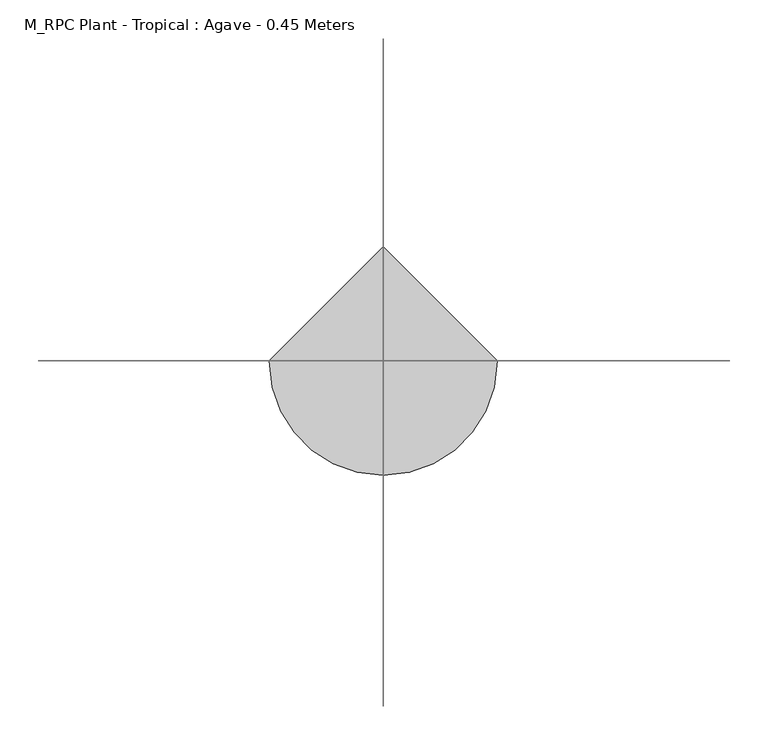
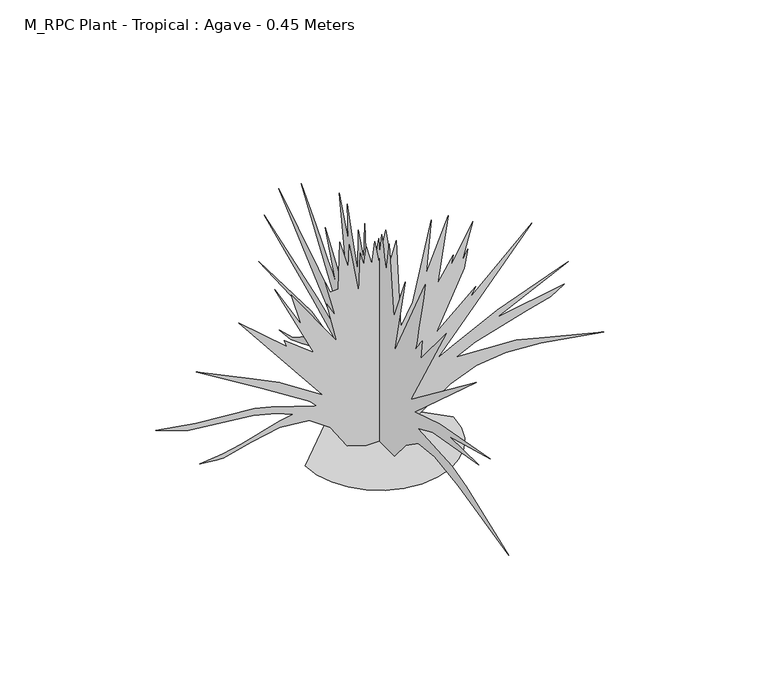
"""IFC4 building model written with IfcOpenShell, lengths in millimetres: geographic element geometry, M_RPC Plant - Tropical : Agave - 0.45 Meters."""

from ifc_helpers import new_model, si_unit, origin, place, context, project, spatial, triangles, source, transform, mapped, element, save


def m_rpc_plant_tropical_agave_0_45_meters_eb57889b(model_context):
    return source(origin(), model_context, "Body", "Tessellation", [
        triangles([(-148.1386958, 0.0, 9.3e-06), (-144.2171964, -33.9885277, 9.3e-06), (-133.048683, -65.2018023, 9.3e-06), (-115.5276685, -92.7450748, 9.3e-06), (-92.5484025, -115.7243407, 9.3e-06), (-65.0051301, -133.2453552, 9.3e-06), (-33.7918577, -144.4138686, 9.3e-06), (0.1966776, -148.335368, 9.3e-06), (34.1851976, -144.4138686, 9.3e-06), (65.3984745, -133.2453552, 9.3e-06), (92.941747, -115.7243407, 9.3e-06), (115.921013, -92.7450748, 9.3e-06), (133.4420274, -65.2018023, 9.3e-06), (144.6105409, -33.9885277, 9.3e-06), (148.5320402, 1.3e-05, 9.3e-06), (0.1966516, 148.335368, 9.3e-06), (-24.3504237, 1.1e-06, 2.5e-06), (-64.1988793, 2e-06, 12.9348607), (-97.895905, 5e-07, 64.0713026), (-140.594189, 5e-07, 94.1593235), (-198.9417449, 2.8e-06, 99.5475756), (-255.4485429, 5.9e-06, 87.7748204), (-311.5910826, 9.2e-06, 73.8080584), (-324.2335885, 9.8e-06, 74.3145591), (-359.378609, 1.11e-05, 77.950311), (-313.1035629, 8.8e-06, 82.7858171), (-277.6960585, 6.8e-06, 90.344322), (-199.7057426, 2e-06, 113.0485866), (-172.7469775, 5e-07, 117.942592), (-204.8844963, 1.2e-06, 130.9928583), (-252.5285358, 2.5e-06, 143.4918682), (-382.9561306, 7.4e-06, 157.5558808), (-447.8461741, 8.9e-06, 179.7488939), (-367.8611217, 6.2e-06, 166.4181305), (-249.0960418, 1.6e-06, 156.7231191), (-216.6905162, 6e-07, 148.7013704), (-125.4831746, -1.6e-06, 119.154591), (-138.0646922, -1.9e-06, 133.1736027), (-234.3990283, -1.3e-06, 193.9569111), (-366.6486231, -4e-07, 275.4877267), (-252.1085396, -2.1e-06, 220.5199336), (-200.6204942, -2.9e-06, 195.5036553), (-113.3644194, -3.3e-06, 138.5448591), (-281.816065, -8.5e-06, 349.4127929), (-184.8657327, -7.8e-06, 265.7927153), (-189.7134928, -8.4e-06, 280.3352324), (-131.5426794, -8.2e-06, 234.2839372), (-209.1037518, -1.44e-05, 395.4653234), (-155.7804623, -1.12e-05, 302.1502344), (-176.3827294, -1.45e-05, 372.4403117), (-85.4908937, -1.07e-05, 242.7671948), (-104.8811618, -1.49e-05, 327.6002798), (-87.9146465, -1.39e-05, 297.3027469), (-108.5169137, -1.76e-05, 374.8628019), (-97.9506527, -1.66e-05, 351.3077717), (-81.76514, -1.74e-05, 351.3277923), (-79.4313889, -2.33e-05, 450.0003668), (-62.2313759, -2.06e-05, 390.7203006), (-60.0411253, -2.35e-05, 437.880358), (-40.6511115, -1.79e-05, 330.02277), (-38.2271089, -2.29e-05, 412.4328197), (-30.9558549, -2.16e-05, 384.5578134), (-26.1083514, -2.4e-05, 422.1278312), (-15.2013409, -2.2e-05, 380.9227881), (-9.1419111, -2.5e-05, 426.9753551), (-0.6586671, -2.27e-05, 380.9227881), (12.6721065, -2.7e-05, 443.9403442), (23.5791135, -2.35e-05, 377.2877993), (34.4861967, -2.62e-05, 413.6428476), (42.9694566, -1.54e-05, 227.0126877), (67.2069761, -1.91e-05, 271.8527196), (104.0335027, -3.03e-05, 433.0253491), (93.8687435, -2.34e-05, 323.9627475), (138.4672839, -3.17e-05, 430.0728404), (116.8945182, -2.27e-05, 294.8777314), (148.4037868, -2.69e-05, 343.3552774), (143.5562902, -2.54e-05, 321.5402573), (187.1843049, -3.2e-05, 400.312811), (165.3703021, -2.65e-05, 322.7527559), (177.4890573, -2.84e-05, 345.7777677), (170.9330439, -2.58e-05, 308.0802504), (114.4707654, -1.64e-05, 190.6558953), (193.2438187, -2.4e-05, 260.9452096), (181.1248092, -2.22e-05, 240.3434511), (305.9494211, -3.46e-05, 355.4727791), (116.8945182, -1.32e-05, 136.120861), (156.175787, -1.61e-05, 155.588123), (236.8716063, -2.2e-05, 195.5036553), (378.6619886, -3.14e-05, 248.8266905), (235.6598525, -2.1e-05, 179.7488939), (371.0494809, -2.83e-05, 203.1156544), (343.871961, -2.62e-05, 186.8916447), (295.8769073, -2.33e-05, 173.2968894), (192.5770716, -1.7e-05, 143.7823665), (154.4632825, -1.42e-05, 125.2138505), (274.4393895, -1.91e-05, 119.154591), (331.2944584, -2.07e-05, 104.4295814), (450.1645283, -2.41e-05, 74.3145591), (324.0894476, -1.98e-05, 94.6895782), (253.5743659, -1.7e-05, 99.5105775), (194.5445751, -1.4e-05, 92.6238249), (142.6707883, -1.05e-05, 72.2130568), (85.3409936, -5.7e-06, 33.5950265), (32.7349455, -1.4e-06, 0.0), (0.196672, 19.7673413, 8.9e-06), (0.1966732, 47.0472873, 9.8e-06), (0.1966747, 67.3315551, 19.7666418), (0.1966772, 98.1250789, 58.1885449), (0.1966793, 130.6278551, 79.4465678), (0.1966812, 171.5303912, 83.5105639), (0.1966824, 205.2991693, 71.7218077), (0.1966844, 267.9552104, 45.114788), (0.1966857, 307.0702466, 29.8075238), (0.1966874, 347.7627846, 24.6271691), (0.1966857, 300.5702436, 38.2485284), (0.1966843, 245.8184439, 73.6468083), (0.1966827, 196.7091595, 96.1225757), (0.196681, 158.7086266, 94.9168263), (0.1966826, 185.5584048, 108.6283349), (0.1966859, 252.0827055, 120.1018443), (0.1966936, 419.0128324, 127.5108488), (0.1966855, 235.0574365, 132.4853544), (0.1966818, 162.3476305, 116.8738436), (0.1966792, 117.5043466, 94.9168263), (0.1966819, 157.4268734, 125.6566015), (0.1966862, 230.1374425, 162.6691225), (0.196696, 399.8753377, 236.7079353), (0.1966859, 214.4554237, 174.9013882), (0.1966819, 145.377618, 145.8161177), (0.1966963, 348.9752832, 323.9627475), (0.1966833, 143.900864, 195.427915), (0.1966945, 270.2027113, 382.1353231), (0.1966926, 244.8639419, 353.83527), (0.1966907, 220.4639232, 326.4102725), (0.1966889, 197.940407, 300.737748), (0.1966873, 178.2316355, 277.6927156), (0.196686, 162.2761232, 258.1477059), (0.1966851, 151.0121214, 242.9834425), (0.1966845, 145.377618, 233.0721834), (0.1966896, 187.793897, 339.7177814), (0.196686, 146.5683701, 279.2777206), (0.1966856, 142.6428648, 273.9577147), (0.1966852, 137.8938633, 268.445206), (0.1966848, 132.4583575, 262.7727143), (0.1966844, 126.4736029, 256.975212), (0.1966839, 120.0768458, 251.0802049), (0.1966835, 113.4055869, 245.1219385), (0.196683, 106.5973361, 239.1316973), (0.1966904, 138.1063594, 442.7278456), (0.1966867, 107.8090899, 361.5328016), (0.196689, 111.4448418, 435.4578315), (0.196687, 96.9023247, 386.9828107), (0.1966838, 73.8763092, 315.4802347), (0.1966864, 72.6643101, 403.9478362), (0.196684, 54.4860456, 353.0502889), (0.1966862, 50.8502891, 430.6103439), (0.1966844, 46.5152885, 378.1328058), (0.1966819, 26.6125221, 322.7527559), (0.1966839, 1.1628534, 429.3978453), (0.1966829, -1.2609561, 399.1003123), (0.1966839, -8.4154066, 443.3628722), (0.1966833, -11.7897339, 429.27536), (0.1966828, -15.0040374, 415.6178361), (0.1966823, -17.8983397, 402.817818), (0.1966818, -20.312591, 391.3078011), (0.1966815, -22.0867923, 381.5153028), (0.1966812, -23.0609175, 373.8703116), (0.196681, -23.0749678, 368.8027794), (0.1966826, -33.9820282, 439.0928567), (0.1966776, -49.7365399, 293.6677398), (0.1966787, -90.9408244, 393.0427969), (0.1966754, -52.1602928, 222.165182), (0.1966767, -160.0183758, 429.3978453), (0.1966761, -153.4961177, 397.6378289), (0.1966754, -147.1613663, 367.0353001), (0.1966749, -141.2021097, 338.7452754), (0.1966744, -135.8058548, 313.9252424), (0.196674, -131.1606078, 293.7327431), (0.1966737, -127.4541026, 279.3227215), (0.1966736, -124.8736006, 271.8527196), (0.1966736, -124.0245972, 269.8952083), (0.1966736, -125.1655977, 270.9177113), (0.1966735, -127.9646002, 274.4252189), (0.1966735, -132.0906019, 279.9202323), (0.1966735, -137.2113559, 286.9052347), (0.1966735, -142.995614, 294.8852345), (0.1966734, -149.1113653, 303.3627512), (0.1966725, -143.0521149, 262.1577082), (0.1966717, -232.7319426, 370.0152781), (0.1966708, -109.1190844, 155.5111291), (0.1966659, -335.7427697, 328.8102714), (0.1966697, -122.4498477, 136.1211063), (0.1966666, -209.7059134, 163.9943868), (0.1966597, -385.1278004, 196.2989011), (0.196665, -242.4269358, 157.9348729), (0.1966604, -345.9302656, 160.358871), (0.1966667, -186.3451482, 131.3988564), (0.1966683, -133.3568582, 108.2475896), (0.1966628, -253.3352089, 100.9760767), (0.1966602, -301.8102479, 87.6453225), (0.1966519, -448.4478453, 30.686524), (0.196661, -273.6277203, 71.7218077), (0.196665, -192.0614054, 83.6695659), (0.1966673, -135.4426048, 77.7298121), (0.1966684, -92.7000739, 48.0972868), (0.1966688, -51.7737929, 6.8e-06), (0.1966702, -18.8243404, 7.8e-06)], [[15, 16, 1], [14, 15, 1], [14, 1, 2], [13, 14, 2], [13, 2, 3], [13, 3, 4], [12, 13, 4], [11, 12, 4], [11, 4, 5], [11, 5, 6], [11, 6, 7], [11, 7, 8], [11, 8, 9], [11, 9, 10], [47, 48, 49], [97, 98, 99], [88, 89, 90], [39, 40, 41], [84, 85, 86], [71, 72, 73], [53, 54, 55], [32, 33, 34], [43, 44, 45], [24, 25, 26], [58, 59, 60], [77, 78, 79], [73, 74, 75], [60, 61, 62], [51, 52, 53], [56, 57, 58], [82, 83, 84], [79, 80, 81], [64, 65, 66], [49, 50, 51], [68, 69, 70], [75, 76, 77], [90, 91, 92], [90, 92, 93], [66, 67, 68], [82, 84, 86], [90, 93, 94], [62, 63, 64], [47, 49, 51], [39, 41, 42], [45, 46, 47], [43, 45, 47], [38, 39, 42], [38, 42, 43], [31, 32, 34], [31, 34, 35], [23, 24, 26], [56, 58, 60], [87, 88, 90], [87, 90, 94], [87, 94, 95], [37, 38, 43], [86, 87, 95], [71, 73, 75], [96, 97, 99], [96, 99, 100], [95, 96, 100], [95, 100, 101], [95, 101, 102], [53, 55, 56], [53, 56, 60], [22, 23, 26], [22, 26, 27], [22, 27, 28], [21, 22, 28], [60, 62, 64], [43, 47, 51], [30, 31, 35], [30, 35, 36], [30, 36, 37], [29, 30, 37], [86, 95, 102], [21, 28, 29], [20, 21, 29], [20, 29, 37], [19, 20, 37], [86, 102, 103], [66, 68, 70], [64, 66, 70], [60, 64, 70], [53, 60, 70], [51, 53, 70], [43, 51, 70], [77, 79, 81], [77, 81, 82], [75, 77, 82], [71, 75, 82], [70, 71, 82], [70, 82, 86], [43, 70, 86], [43, 86, 103], [43, 103, 104], [43, 104, 17], [43, 17, 18], [43, 18, 19], [43, 19, 37], [120, 121, 122], [193, 194, 195], [190, 191, 192], [126, 127, 128], [155, 156, 157], [131, 132, 133], [200, 201, 202], [113, 114, 115], [195, 196, 197], [129, 130, 131], [131, 133, 134], [170, 171, 172], [188, 189, 190], [131, 134, 135], [148, 149, 150], [139, 140, 141], [131, 135, 136], [150, 151, 152], [168, 169, 170], [172, 173, 174], [131, 136, 137], [158, 159, 160], [172, 174, 175], [131, 137, 138], [153, 154, 155], [131, 138, 139], [172, 175, 176], [160, 161, 162], [172, 176, 177], [186, 187, 188], [172, 177, 178], [112, 113, 115], [112, 115, 116], [111, 112, 116], [111, 116, 117], [160, 162, 163], [172, 178, 179], [172, 179, 180], [172, 180, 181], [139, 141, 142], [193, 195, 197], [185, 186, 188], [192, 193, 197], [192, 197, 198], [155, 157, 158], [150, 152, 153], [148, 150, 153], [139, 142, 143], [199, 200, 202], [119, 120, 122], [119, 122, 123], [118, 119, 123], [199, 202, 203], [198, 199, 203], [198, 203, 204], [184, 185, 188], [110, 111, 117], [110, 117, 118], [109, 110, 118], [160, 163, 164], [118, 123, 124], [109, 118, 124], [139, 143, 144], [125, 126, 128], [125, 128, 129], [183, 184, 188], [139, 144, 145], [153, 155, 158], [108, 109, 124], [139, 145, 146], [160, 164, 165], [158, 160, 165], [158, 165, 166], [158, 166, 167], [158, 167, 168], [158, 168, 170], [182, 183, 188], [124, 125, 129], [182, 188, 190], [181, 182, 190], [172, 181, 190], [139, 146, 147], [131, 139, 147], [131, 147, 148], [158, 170, 172], [153, 158, 172], [148, 153, 172], [198, 204, 205], [131, 148, 172], [129, 131, 172], [124, 129, 172], [124, 172, 190], [108, 124, 190], [107, 108, 190], [106, 107, 190], [105, 106, 190], [207, 105, 190], [206, 207, 190], [205, 206, 190], [198, 205, 190], [192, 198, 190]], closed=False),
    ])


if __name__ == "__main__":
    model = new_model("IFC4")
    model_context = context("Model", 3, world=origin())
    ifc_project = project(units=[si_unit("LENGTHUNIT", "METRE", prefix="MILLI")], contexts=[model_context])
    site = spatial("IfcSite", under=ifc_project)
    building = spatial("IfcBuilding", under=site)
    placement = place(None, origin())
    m_rpc_plant_tropical_agave_0_45_meters_shape = m_rpc_plant_tropical_agave_0_45_meters_eb57889b(model_context)
    element("IfcGeographicElement", 1, ObjectType="M_RPC Plant - Tropical : Agave - 0.45 Meters", at=placement, inside=building, context=model_context, shape_type="MappedRepresentation", body=[
        mapped(m_rpc_plant_tropical_agave_0_45_meters_shape, transform((0.0, 0.0, 0.0), x_axis=(1.0, 0.0, 0.0), y_axis=(0.0, 1.0, 0.0), z_axis=(0.0, 0.0, 1.0))),
    ])
    save(model, "model.ifc")

# Revit data of these elements
# Type "M_RPC Plant - Tropical : Agave - 0.45 Meters"
#   built-in parameter 1005198 = "{2, 15},{39, RPC-16-G1GJ-63FX-7K5P-N000-ST1L-LVER-AU},{1, 0},{1, 0},{2, 13},{1, 8},{5, Color},{1, 0},{1, 0},{3, 0.8},{3, 0.8},{3, 0.8},{1, 8},{7, BBoxMin},{1, 0},{1, 0},{1, 0},{1, 0},{1, 0},{1, 8},{7, BBoxMax},{1, 0},{1, 0},{1, 0},{1, 0},{1, 0},{2, 11},{9, RPCTypeId},{1, 0},{1, 0},{39, RPC-16-G1GJ-63FX-7K5P-N000-ST1L-LVER-AU},{1, 6},{14, RPCPlantHeight},{1, 0},{1, 0},{7, 1.47638},{2, 11},{7, keyword},{1, 0},{1, 0},{35, :RPCs:Plants [General]:Geometry:RPC},{2, 11},{8, category},{1, 0},{1, 0},{16, Plants [General]},{2, 11},{12, LocalizedUID},{1, 0},{1, 0},{5, Agave},{2, 14},{6, Height},{1, 0},{1, 0},{7, 1.47638},{1, 2},{16, Cast Reflections},{1, 0},{1, 0},{1, 0},{1, 2},{12, Cast Shadows},{1, 0},{1, 0},{1, 1},{1, 2},{9, Lock View},{1, 0},{1, 0},{1, 0},{1, 4},{5, ViewC},{1, 0},{1, 0},{1, 0},{21, assetlibrary_base.fbx},{1, 5},"
#   built-in parameter 1005195 = "RPC-16-G1GJ-63FX-7K5P-N000-ST1L-LVER-AU"
#   Type Comments = "Agave"
#   Height = 450 mm
#   Description = (empty or 0)
#   Default Elevation = 0
